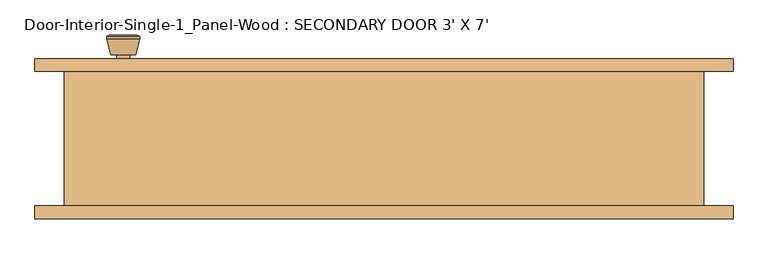
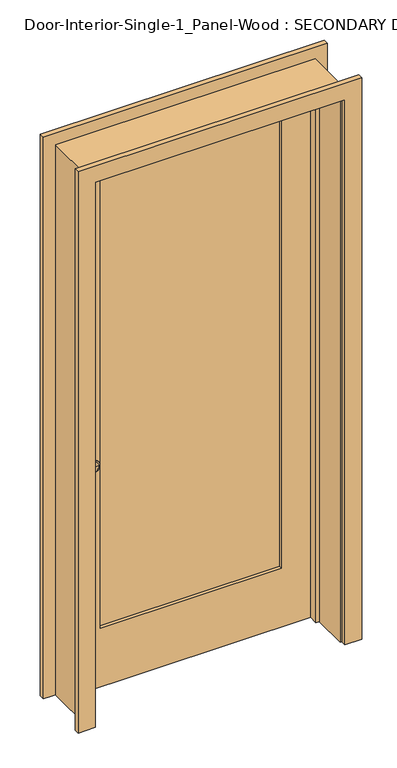
"""IFC4 building model written with IfcOpenShell, lengths in millimetres: door geometry, Door-Interior-Single-1_Panel-Wood : SECONDARY DOOR 3' X 7'."""

from ifc_helpers import new_model, si_unit, point, frame, frame_2d, origin, place, context, project, spatial, polyline, circle_curve, trimmed, segment, composite_curve, outline, extrude, faceted_brep, source, transform, mapped, element, save
from ifc_brep_helpers import plane_surface, cylinder_surface, revolved_surface, advanced_brep


def door_interior_single_1_panel_wood_secondary_door_3_x_7_9c4ddfbd(model_context):
    return source(origin(), model_context, "Body", "SolidModel", [
        advanced_brep(
        [(-393.7, 57.5, 914.4), (-383.7, 57.5, 914.4), (-403.7, 57.5, 914.4), (-373.2241324, 8.5, 914.4), (-393.7, 8.5, 914.4), (-414.1758676, 8.5, 914.4), (-368.7, 10.3278681, 914.4), (-418.7, 10.3278681, 914.4), (-368.7, 13.7915463, 914.4), (-418.7, 13.7915463, 914.4), (-375.063764, 38.5, 914.4), (-412.336236, 38.5, 914.4), (-383.7, 38.5, 914.4), (-403.7, 38.5, 914.4)],
        [
            (0, 1),
            (1, 2, circle_curve(frame((-393.7, 57.5, 914.4), z_axis=(0.0, 1.0, 0.0), x_axis=(-1.0, 0.0, 0.0)), 10.0)),
            (2, 0),
            (2, 1, circle_curve(frame((-393.7, 57.5, 914.4), z_axis=(0.0, 1.0, 0.0), x_axis=(-1.0, 0.0, 0.0)), 10.0)),
            (3, 4),
            (4, 5),
            (5, 3, circle_curve(frame((-393.7, 8.5, 914.4), z_axis=(0.0, -1.0, 0.0), x_axis=(-1.0, 0.0, 0.0)), 20.4758676)),
            (3, 5, circle_curve(frame((-393.7, 8.5, 914.4), z_axis=(0.0, -1.0, 0.0), x_axis=(-1.0, 0.0, 0.0)), 20.4758676)),
            (6, 3),
            (5, 7),
            (7, 6, circle_curve(frame((-393.7, 10.3278681, 914.4), z_axis=(0.0, -1.0, 0.0), x_axis=(-1.0, 0.0, 0.0)), 25.0)),
            (6, 7, circle_curve(frame((-393.7, 10.3278681, 914.4), z_axis=(0.0, -1.0, 0.0), x_axis=(-1.0, 0.0, 0.0)), 25.0)),
            (8, 6),
            (7, 9),
            (9, 8, circle_curve(frame((-393.7, 13.7915463, 914.4), z_axis=(0.0, -1.0, 0.0), x_axis=(-1.0, 0.0, 0.0)), 25.0)),
            (8, 9, circle_curve(frame((-393.7, 13.7915463, 914.4), z_axis=(0.0, -1.0, 0.0), x_axis=(-1.0, 0.0, 0.0)), 25.0)),
            (10, 8),
            (9, 11),
            (11, 10, circle_curve(frame((-393.7, 38.5, 914.4), z_axis=(0.0, -1.0, 0.0), x_axis=(-1.0, 0.0, 0.0)), 18.636236)),
            (10, 11, circle_curve(frame((-393.7, 38.5, 914.4), z_axis=(0.0, -1.0, 0.0), x_axis=(-1.0, 0.0, 0.0)), 18.636236)),
            (12, 10),
            (11, 13),
            (13, 12, circle_curve(frame((-393.7, 38.5, 914.4), z_axis=(0.0, -1.0, 0.0), x_axis=(-1.0, 0.0, 0.0)), 10.0)),
            (12, 13, circle_curve(frame((-393.7, 38.5, 914.4), z_axis=(0.0, -1.0, 0.0), x_axis=(-1.0, 0.0, 0.0)), 10.0)),
            (1, 12),
            (13, 2),
        ],
        [
            plane_surface(frame((-393.7, 57.5, 914.4), z_axis=(0.0, 1.0, 0.0), x_axis=(-1.0, 0.0, 0.0))),
            plane_surface(frame((-393.7, 8.5, 914.4), z_axis=(0.0, -1.0, 0.0), x_axis=(-1.0, 0.0, 0.0))),
            revolved_surface(polyline([(-414.1758676, 8.5, 914.4), (-418.7, 10.3278681, 914.4)]), (-393.7, 57.5, 914.4), (0.0, 1.0, 0.0)),
            cylinder_surface(frame((-393.7, 57.5, 914.4), z_axis=(0.0, 1.0, 0.0), x_axis=(-1.0, 0.0, 0.0)), 25.0),
            revolved_surface(polyline([(-418.7, 13.7915463, 914.4), (-412.336236, 38.5, 914.4)]), (-393.7, 57.5, 914.4), (0.0, 1.0, 0.0)),
            plane_surface(frame((-393.7, 38.5, 914.4), z_axis=(0.0, 1.0, 0.0), x_axis=(-1.0, 0.0, 0.0))),
            cylinder_surface(frame((-393.7, 57.5, 914.4), z_axis=(0.0, 1.0, 0.0), x_axis=(-1.0, 0.0, 0.0)), 10.0),
        ],
        [
            (0, [[1, 2, 3]]),
            (0, [[-3, 4, -1]]),
            (1, [[5, 6, 7]]),
            (1, [[-6, -5, 8]]),
            (2, [[9, -7, 10, 11]]),
            (2, [[-10, -8, -9, 12]]),
            (3, [[13, -11, 14, 15]]),
            (3, [[-14, -12, -13, 16]]),
            (4, [[17, -15, 18, 19]]),
            (4, [[-18, -16, -17, 20]]),
            (5, [[21, -19, 22, 23]]),
            (5, [[-22, -20, -21, 24]]),
            (6, [[25, -23, 26, -2]]),
            (6, [[-26, -24, -25, -4]]),
        ],
    ),
        extrude(outline(composite_curve([segment(trimmed(circle_curve(frame_2d((914.4, -393.7)), 30.0), [point((914.4, -423.7))], [point((914.4, -363.7))], False, "CARTESIAN"), True, "CONTINUOUS"), segment(trimmed(circle_curve(frame_2d((914.4, -393.7)), 30.0), [point((914.4, -363.7))], [point((914.4, -423.7))], False, "CARTESIAN"), True, "CONTINUOUS")], self_intersect=False)), frame((0.0, 57.5, 0.0), z_axis=(0.0, 1.0, 0.0), x_axis=(0.0, 0.0, 1.0)), (0.0, 0.0, 1.0), 6.0),
        advanced_brep(
        [(-393.7, 104.425, 914.4), (-403.7, 104.425, 914.4), (-383.7, 104.425, 914.4), (-373.2241324, 153.425, 914.4), (-414.1758676, 153.425, 914.4), (-393.7, 153.425, 914.4), (-368.7, 151.5971319, 914.4), (-418.7, 151.5971319, 914.4), (-368.7, 148.1334537, 914.4), (-418.7, 148.1334537, 914.4), (-375.063764, 123.425, 914.4), (-412.336236, 123.425, 914.4), (-383.7, 123.425, 914.4), (-403.7, 123.425, 914.4)],
        [
            (0, 1),
            (1, 2, circle_curve(frame((-393.7, 104.425, 914.4), z_axis=(0.0, -1.0, 0.0), x_axis=(-1.0, 0.0, 0.0)), 10.0)),
            (2, 0),
            (2, 1, circle_curve(frame((-393.7, 104.425, 914.4), z_axis=(0.0, -1.0, 0.0), x_axis=(-1.0, 0.0, 0.0)), 10.0)),
            (3, 4, circle_curve(frame((-393.7, 153.425, 914.4), z_axis=(0.0, 1.0, 0.0), x_axis=(-1.0, 0.0, 0.0)), 20.4758676)),
            (4, 5),
            (5, 3),
            (4, 3, circle_curve(frame((-393.7, 153.425, 914.4), z_axis=(0.0, 1.0, 0.0), x_axis=(-1.0, 0.0, 0.0)), 20.4758676)),
            (6, 7, circle_curve(frame((-393.7, 151.5971319, 914.4), z_axis=(0.0, 1.0, 0.0), x_axis=(-1.0, 0.0, 0.0)), 25.0)),
            (7, 4),
            (3, 6),
            (7, 6, circle_curve(frame((-393.7, 151.5971319, 914.4), z_axis=(0.0, 1.0, 0.0), x_axis=(-1.0, 0.0, 0.0)), 25.0)),
            (8, 9, circle_curve(frame((-393.7, 148.1334537, 914.4), z_axis=(0.0, 1.0, 0.0), x_axis=(-1.0, 0.0, 0.0)), 25.0)),
            (9, 7),
            (6, 8),
            (9, 8, circle_curve(frame((-393.7, 148.1334537, 914.4), z_axis=(0.0, 1.0, 0.0), x_axis=(-1.0, 0.0, 0.0)), 25.0)),
            (10, 11, circle_curve(frame((-393.7, 123.425, 914.4), z_axis=(0.0, 1.0, 0.0), x_axis=(-1.0, 0.0, 0.0)), 18.636236)),
            (11, 9),
            (8, 10),
            (11, 10, circle_curve(frame((-393.7, 123.425, 914.4), z_axis=(0.0, 1.0, 0.0), x_axis=(-1.0, 0.0, 0.0)), 18.636236)),
            (12, 13, circle_curve(frame((-393.7, 123.425, 914.4), z_axis=(0.0, 1.0, 0.0), x_axis=(-1.0, 0.0, 0.0)), 10.0)),
            (13, 11),
            (10, 12),
            (13, 12, circle_curve(frame((-393.7, 123.425, 914.4), z_axis=(0.0, 1.0, 0.0), x_axis=(-1.0, 0.0, 0.0)), 10.0)),
            (1, 13),
            (12, 2),
        ],
        [
            plane_surface(frame((-393.7, 104.425, 914.4), z_axis=(0.0, -1.0, 0.0), x_axis=(-1.0, 0.0, 0.0))),
            plane_surface(frame((-393.7, 153.425, 914.4), z_axis=(0.0, 1.0, 0.0), x_axis=(-1.0, 0.0, 0.0))),
            revolved_surface(polyline([(-414.1758676, 153.425, 914.4), (-418.7, 151.5971319, 914.4)]), (-393.7, 104.425, 914.4), (0.0, -1.0, 0.0)),
            cylinder_surface(frame((-393.7, 104.425, 914.4), z_axis=(0.0, -1.0, 0.0), x_axis=(-1.0, 0.0, 0.0)), 25.0),
            revolved_surface(polyline([(-418.7, 148.1334537, 914.4), (-412.336236, 123.425, 914.4)]), (-393.7, 104.425, 914.4), (0.0, -1.0, 0.0)),
            plane_surface(frame((-393.7, 123.425, 914.4), z_axis=(0.0, -1.0, 0.0), x_axis=(-1.0, 0.0, 0.0))),
            cylinder_surface(frame((-393.7, 104.425, 914.4), z_axis=(0.0, -1.0, 0.0), x_axis=(-1.0, 0.0, 0.0)), 10.0),
        ],
        [
            (0, [[1, 2, 3]]),
            (0, [[-3, 4, -1]]),
            (1, [[5, 6, 7]]),
            (1, [[8, -7, -6]]),
            (2, [[9, 10, -5, 11]]),
            (2, [[12, -11, -8, -10]]),
            (3, [[13, 14, -9, 15]]),
            (3, [[16, -15, -12, -14]]),
            (4, [[17, 18, -13, 19]]),
            (4, [[20, -19, -16, -18]]),
            (5, [[21, 22, -17, 23]]),
            (5, [[24, -23, -20, -22]]),
            (6, [[-2, 25, -21, 26]]),
            (6, [[-4, -26, -24, -25]]),
        ],
    ),
        extrude(outline(composite_curve([segment(trimmed(circle_curve(frame_2d((914.4, -393.7)), 30.0), [point((914.4, -423.7))], [point((914.4, -363.7))], False, "CARTESIAN"), True, "CONTINUOUS"), segment(trimmed(circle_curve(frame_2d((914.4, -393.7)), 30.0), [point((914.4, -363.7))], [point((914.4, -423.7))], False, "CARTESIAN"), True, "CONTINUOUS")], self_intersect=False)), frame((0.0, 98.425, 0.0), z_axis=(0.0, 1.0, 0.0), x_axis=(0.0, 0.0, 1.0)), (0.0, 0.0, 1.0), 6.0),
        faceted_brep([(482.6, 98.425, 0.0), (482.6, -104.775, 0.0), (457.2, -104.775, 0.0), (457.2, 28.575, 0.0), (444.5, 28.575, 0.0), (444.5, 63.5, 0.0), (457.2, 63.5, 0.0), (457.2, 98.425, 0.0), (482.6, 98.425, 2159.0), (482.6, -104.775, 2159.0), (-482.6, -104.775, 2159.0), (-482.6, -104.775, 0.0), (-457.2, -104.775, 0.0), (-457.2, -104.775, 2133.6), (457.2, -104.775, 2133.6), (457.2, 28.575, 2133.6), (-457.2, 28.575, 2133.6), (-457.2, 28.575, 0.0), (-444.5, 28.575, 0.0), (-444.5, 28.575, 2120.9), (444.5, 28.575, 2120.9), (444.5, 63.5, 2120.9), (-444.5, 63.5, 2120.9), (-444.5, 63.5, 0.0), (-457.2, 63.5, 0.0), (-457.2, 63.5, 2133.6), (457.2, 63.5, 2133.6), (457.2, 98.425, 2133.6), (-457.2, 98.425, 2133.6), (-457.2, 98.425, 0.0), (-482.6, 98.425, 0.0), (-482.6, 98.425, 2159.0)], [[[0, 1, 2, 3, 4, 5, 6, 7]], [[1, 0, 8, 9]], [[2, 1, 9, 10, 11, 12, 13, 14]], [[3, 2, 14, 15]], [[4, 3, 15, 16, 17, 18, 19, 20]], [[5, 4, 20, 21]], [[6, 5, 21, 22, 23, 24, 25, 26]], [[7, 6, 26, 27]], [[0, 7, 27, 28, 29, 30, 31, 8]], [[9, 8, 31, 10]], [[15, 14, 13, 16]], [[21, 20, 19, 22]], [[27, 26, 25, 28]], [[30, 29, 24, 23, 18, 17, 12, 11]], [[10, 31, 30, 11]], [[16, 13, 12, 17]], [[22, 19, 18, 23]], [[28, 25, 24, 29]]]),
        extrude(outline(polyline([(2133.6, -457.2), (0.0, -457.2), (0.0, 457.2), (2133.6, 457.2), (2133.6, -457.2)]), holes=[polyline([(2014.5375, -336.55), (2014.5375, 336.55), (231.775, 336.55), (231.775, -336.55), (2014.5375, -336.55)])]), frame((0.0, 63.5, 0.0), z_axis=(0.0, 1.0, 0.0), x_axis=(0.0, 0.0, 1.0)), (0.0, 0.0, 1.0), 34.925),
        extrude(outline(polyline([(336.55, 75.1416667), (-336.55, 75.1416667), (-336.55, 86.7833333), (336.55, 86.7833333), (336.55, 75.1416667)])), frame((0.0, 0.0, 231.775), z_axis=(0.0, 0.0, 1.0), x_axis=(1.0, 0.0, 0.0)), (0.0, 0.0, 1.0), 1782.7625),
        extrude(outline(polyline([(0.0, 463.55), (0.0, 527.05), (2203.45, 527.05), (2203.45, -527.05), (0.0, -527.05), (0.0, -463.55), (2139.95, -463.55), (2139.95, 463.55), (0.0, 463.55)])), frame((0.0, 98.425, 0.0), z_axis=(0.0, 1.0, 0.0), x_axis=(0.0, 0.0, 1.0)), (0.0, 0.0, 1.0), 19.05),
        extrude(outline(polyline([(0.0, 463.55), (0.0, 527.05), (2203.45, 527.05), (2203.45, -527.05), (0.0, -527.05), (0.0, -463.55), (2139.95, -463.55), (2139.95, 463.55), (0.0, 463.55)])), frame((0.0, -123.825, 0.0), z_axis=(0.0, 1.0, 0.0), x_axis=(0.0, 0.0, 1.0)), (0.0, 0.0, 1.0), 19.05),
    ])


if __name__ == "__main__":
    model = new_model("IFC4")
    model_context = context("Model", 3, world=origin())
    ifc_project = project(units=[si_unit("LENGTHUNIT", "METRE", prefix="MILLI")], contexts=[model_context])
    site = spatial("IfcSite", under=ifc_project)
    building = spatial("IfcBuilding", under=site)
    placement = place(None, origin())
    door_interior_single_1_panel_wood_secondary_door_3_x_7_shape = door_interior_single_1_panel_wood_secondary_door_3_x_7_9c4ddfbd(model_context)
    element("IfcDoor", 1, ObjectType="Door-Interior-Single-1_Panel-Wood : SECONDARY DOOR 3' X 7'", at=placement, inside=building, context=model_context, shape_type="MappedRepresentation", body=[
        mapped(door_interior_single_1_panel_wood_secondary_door_3_x_7_shape, transform((0.0, 0.0, 0.0), x_axis=(1.0, 0.0, 0.0), y_axis=(0.0, 1.0, 0.0), z_axis=(0.0, 0.0, 1.0))),
    ])
    save(model, "model.ifc")

# Revit data of these elements
# Type "Door-Interior-Single-1_Panel-Wood : SECONDARY DOOR 3' X 7'"
#   Type Mark = "11"
#   Assembly Code = "C1020300"
#   Analytic Construction = "Wooden"
#   Top Rail = 0' - 4 11/16"
#   Thickness = 0' - 1 3/8"
#   Thermal Resistance (R) = 2.5876 (h·ft²·°F)/BTU
#   Swing Angle [instance default] = 90.00°
#   Stiles = 0' - 4 3/4"
#   Rough Width = 3' - 2"
#   Rough Height = 7' - 1"
#   Height = 7' - 0"
#   Width = 3' - 0"
#   Heat Transfer Coefficient (U) = 0.3865 BTU/(h·ft²·°F)
#   Bottom Rail = 0' - 9 1/8"
#   Trim Material = Cherry
#   Panel Material = Cherry
#   Frame Material = Cherry
#   Door Handle Material = Aluminum
#   Visual Light Transmittance = 0
#   Solar Heat Gain Coefficient = 0
#   Wall Closure = (empty or 0)
#   Function = (empty or 0)
# Element 1 (IfcDoor, "Door-Interior-Single-1_Panel-Wood : SECONDARY DOOR 3' X 7'")
#   Materials on its faces: "Cherry", "Aluminum"
# Materials
#   "Cherry": class "Wood", colour RGB 226 177 128, transparency 0, Description = "Prunus Serotina", Cost = 0
#   "Aluminum": class "Metal", colour RGB 247 247 247, transparency 0, Description = "Aluminum 6061", Cost = 0
